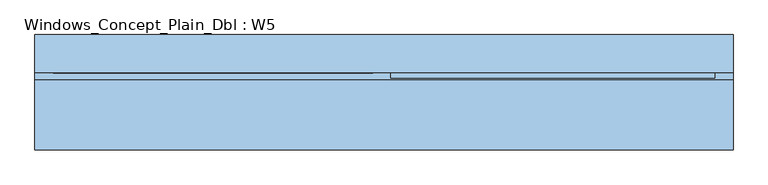
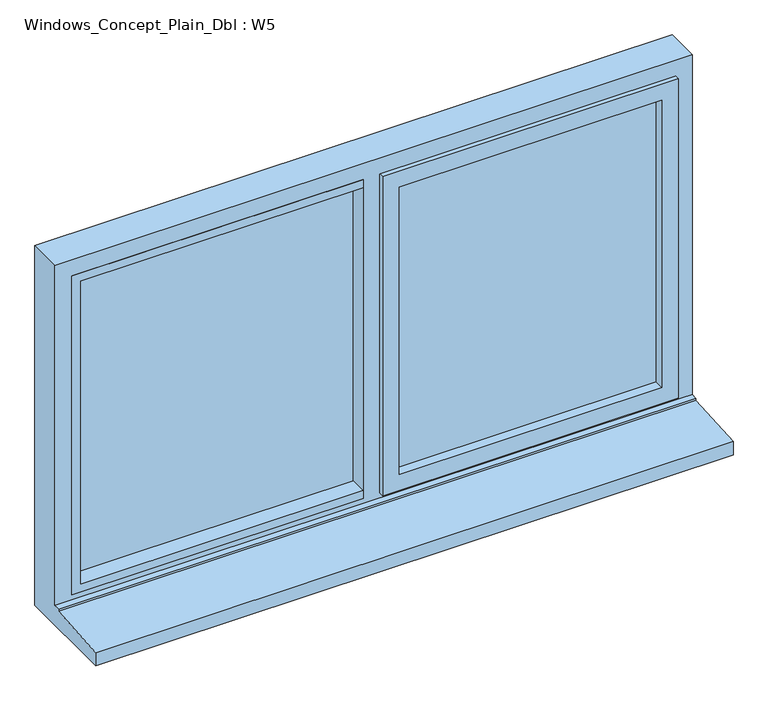
"""IFC4 building model written with IfcOpenShell, lengths in millimetres: window geometry, Windows_Concept_Plain_Dbl : W5."""

from ifc_helpers import new_model, si_unit, frame, origin, place, context, project, spatial, polyline, outline, extrude, faceted_brep, source, transform, mapped, element, save


def windows_concept_plain_dbl_w5_572de7b6(model_context):
    return source(origin(), model_context, "Body", "SolidModel", [
        faceted_brep([(-270.0, 37.9634322, 2070.0), (-270.0, 37.9634322, 1263.0), (-270.0, -38.5835732, 1263.0), (-270.0, -38.5835732, 2070.0), (-230.0, 8.9634322, 2030.0), (-230.0, 8.9634322, 1303.0), (-230.0, 37.9634322, 1303.0), (-230.0, 37.9634322, 2030.0), (-240.0, -15.0365678, 2040.0), (-240.0, -15.0365678, 1293.0), (-240.0, 8.9634322, 1293.0), (-240.0, 8.9634322, 2040.0), (-230.0, -38.5835732, 2030.0), (-230.0, -38.5835732, 1303.0), (-230.0, -15.0365678, 1303.0), (-230.0, -15.0365678, 2030.0), (437.0, 37.9634322, 1263.0), (437.0, -38.5835732, 1263.0), (397.0, 8.9634322, 1303.0), (397.0, 37.9634322, 1303.0), (407.0, -15.0365678, 1293.0), (407.0, 8.9634322, 1293.0), (397.0, -38.5835732, 1303.0), (397.0, -15.0365678, 1303.0), (437.0, 37.9634322, 2070.0), (437.0, -38.5835732, 2070.0), (397.0, 8.9634322, 2030.0), (397.0, 37.9634322, 2030.0), (407.0, -15.0365678, 2040.0), (407.0, 8.9634322, 2040.0), (397.0, -38.5835732, 2030.0), (397.0, -15.0365678, 2030.0)], [[[0, 1, 2, 3]], [[4, 5, 6, 7]], [[8, 9, 10, 11]], [[12, 13, 14, 15]], [[1, 16, 17, 2]], [[5, 18, 19, 6]], [[9, 20, 21, 10]], [[13, 22, 23, 14]], [[16, 24, 25, 17]], [[18, 26, 27, 19]], [[20, 28, 29, 21]], [[22, 30, 31, 23]], [[3, 2, 17, 25], [13, 12, 30, 22]], [[24, 0, 3, 25]], [[1, 0, 24, 16], [7, 6, 19, 27]], [[26, 4, 7, 27]], [[11, 10, 21, 29], [5, 4, 26, 18]], [[28, 8, 11, 29]], [[9, 8, 28, 20], [15, 14, 23, 31]], [[30, 12, 15, 31]]]),
        extrude(outline(polyline([(2070.0, -310.0), (2070.0, -1007.0), (1263.0, -1007.0), (1263.0, -310.0), (1283.0, -310.0), (1283.0, -987.0), (2050.0, -987.0), (2050.0, -310.0), (2070.0, -310.0)])), frame((0.0, -27.0365678, 0.0), z_axis=(0.0, 1.0, 0.0), x_axis=(0.0, 0.0, 1.0)), (0.0, 0.0, 1.0), 41.0),
        faceted_brep([(477.0, 55.9634322, 2110.0), (477.0, 55.9634322, 1200.0), (-1047.0, 55.9634322, 1200.0), (-1047.0, 55.9634322, 2110.0), (417.0, 55.9634322, 2050.0), (-252.0, 55.9634322, 2050.0), (-252.0, 55.9634322, 1275.0), (417.0, 55.9634322, 1275.0), (-310.0, 55.9634322, 2050.0), (-987.0, 55.9634322, 2050.0), (-987.0, 55.9634322, 1275.0), (-310.0, 55.9634322, 1275.0), (-1047.0, -195.9565678, 1200.0), (-1047.0, -195.9565678, 1233.8088847), (-1047.0, -42.0365678, 1244.7449676), (-1047.0, -42.0365678, 1249.68767), (-1047.0, -27.0365678, 1251.0), (-1047.0, -27.0365678, 2110.0), (477.0, -27.0365678, 1251.0), (477.0, -27.0365678, 2110.0), (-1007.0, -27.0365678, 2070.0), (-310.0, -27.0365678, 2070.0), (-310.0, -27.0365678, 1263.0), (-1007.0, -27.0365678, 1263.0), (-270.0, -27.0365678, 2070.0), (437.0, -27.0365678, 2070.0), (437.0, -27.0365678, 1263.0), (-270.0, -27.0365678, 1263.0), (-1007.0, 37.9634322, 1263.0), (-1007.0, 37.9634322, 2070.0), (-300.0, 37.9634322, 1263.0), (-300.0, 37.9634322, 2070.0), (-310.0, 37.9634322, 2050.0), (-310.0, 37.9634322, 1275.0), (-987.0, 37.9634322, 1275.0), (-987.0, 37.9634322, 2050.0), (-270.0, 37.9634322, 2070.0), (-270.0, 37.9634322, 1263.0), (437.0, 37.9634322, 1263.0), (437.0, 37.9634322, 2070.0), (417.0, 37.9634322, 2050.0), (417.0, 37.9634322, 1275.0), (-252.0, 37.9634322, 1275.0), (-252.0, 37.9634322, 2050.0), (-300.0, 13.9634322, 2070.0), (-310.0, 13.9634322, 2070.0), (477.0, -42.0365678, 1249.68767), (477.0, -42.0365678, 1244.7449676), (477.0, -195.9565678, 1233.8088847), (477.0, -195.9565678, 1200.0), (-300.0, 13.9634322, 1263.0), (-310.0, 13.9634322, 1263.0)], [[[0, 1, 2, 3], [4, 5, 6, 7], [8, 9, 10, 11]], [[2, 12, 13, 14, 15, 16, 17, 3]], [[16, 18, 19, 17], [20, 21, 22, 23], [24, 25, 26, 27]], [[23, 28, 29, 20]], [[29, 28, 30, 31], [32, 33, 34, 35]], [[36, 37, 38, 39], [40, 41, 42, 43]], [[35, 34, 10, 9]], [[3, 17, 19, 0]], [[25, 24, 36, 39]], [[29, 31, 44, 45, 21, 20]], [[9, 8, 32, 35]], [[40, 43, 5, 4]], [[18, 46, 47, 48, 49, 1, 0, 19]], [[25, 39, 38, 26]], [[4, 7, 41, 40]], [[44, 31, 30, 50]], [[50, 51, 45, 44]], [[51, 22, 21, 45]], [[27, 37, 36, 24]], [[43, 42, 6, 5]], [[8, 11, 33, 32]], [[49, 12, 2, 1]], [[48, 13, 12, 49]], [[47, 14, 13, 48]], [[46, 15, 14, 47]], [[18, 16, 15, 46]], [[26, 38, 37, 27]], [[22, 51, 50, 30, 28, 23]], [[6, 42, 41, 7]], [[33, 11, 10, 34]]]),
        extrude(outline(polyline([(-1007.0, 13.9634322), (-1007.0, 37.9634322), (-300.0, 37.9634322), (-300.0, 13.9634322), (-1007.0, 13.9634322)])), frame((0.0, 0.0, 1263.0), z_axis=(0.0, 0.0, 1.0), x_axis=(1.0, 0.0, 0.0)), (0.0, 0.0, 1.0), 807.0),
        extrude(outline(polyline([(407.0, 8.9634322), (407.0, -15.0365678), (-240.0, -15.0365678), (-240.0, 8.9634322), (407.0, 8.9634322)])), frame((0.0, 0.0, 1293.0), z_axis=(0.0, 0.0, 1.0), x_axis=(1.0, 0.0, 0.0)), (0.0, 0.0, 1.0), 747.0),
    ])


if __name__ == "__main__":
    model = new_model("IFC4")
    model_context = context("Model", 3, world=origin())
    ifc_project = project(units=[si_unit("LENGTHUNIT", "METRE", prefix="MILLI")], contexts=[model_context])
    site = spatial("IfcSite", under=ifc_project)
    building = spatial("IfcBuilding", under=site)
    placement = place(None, origin())
    windows_concept_plain_dbl_w5_shape = windows_concept_plain_dbl_w5_572de7b6(model_context)
    element("IfcWindow", 1, ObjectType="Windows_Concept_Plain_Dbl : W5", at=placement, inside=building, context=model_context, shape_type="MappedRepresentation", body=[
        mapped(windows_concept_plain_dbl_w5_shape, transform((0.0, 0.0, 0.0), x_axis=(1.0, 0.0, 0.0), y_axis=(0.0, 1.0, 0.0), z_axis=(0.0, 0.0, 1.0))),
    ])
    save(model, "model.ifc")

# Revit data of these elements
# Type "Windows_Concept_Plain_Dbl : W5"
#   Type Mark = "60"
#   Operation = "DoublePanelVertical"
#   Construction Type Id = "GSP4R"
#   Manufacturer = "Revit"
#   Keynote = "L10"
#   Analytic Construction = "1/8 in Pilkington single glazing"
#   Visual Light Transmittance = 0.9
#   Solar Heat Gain Coefficient = 0.78
#   Rough Width = 1524 mm
#   Rough Height = 910 mm
#   Height = 910 mm
#   Width = 1524 mm
#   Heat Transfer Coefficient (U) = 3.6886 W/(m²·K)
#   FrameOffset - External = 50 mm
#   Default Head Height = 2110 mm
#   Vis - Cavity Closers = yes
#   Define Thermal Properties by = 1
#   Material Trim = Window Frame
#   Material Glass = Glass
#   Material Frame = Window Frame
#   Wall Closure = (empty or 0)
# Element 1 (IfcWindow, "Windows_Concept_Plain_Dbl : W5")
#   Materials on its faces: "Window Frame", "Glass"
# Materials
#   "Window Frame": colour RGB 249 249 249, transparency 0, Keynote = "L10", Cost = 0
#   "Glass": class "Glass", colour RGB 0 128 192, transparency 0.9, Description = "Soda Lime Glass", Cost = 0
